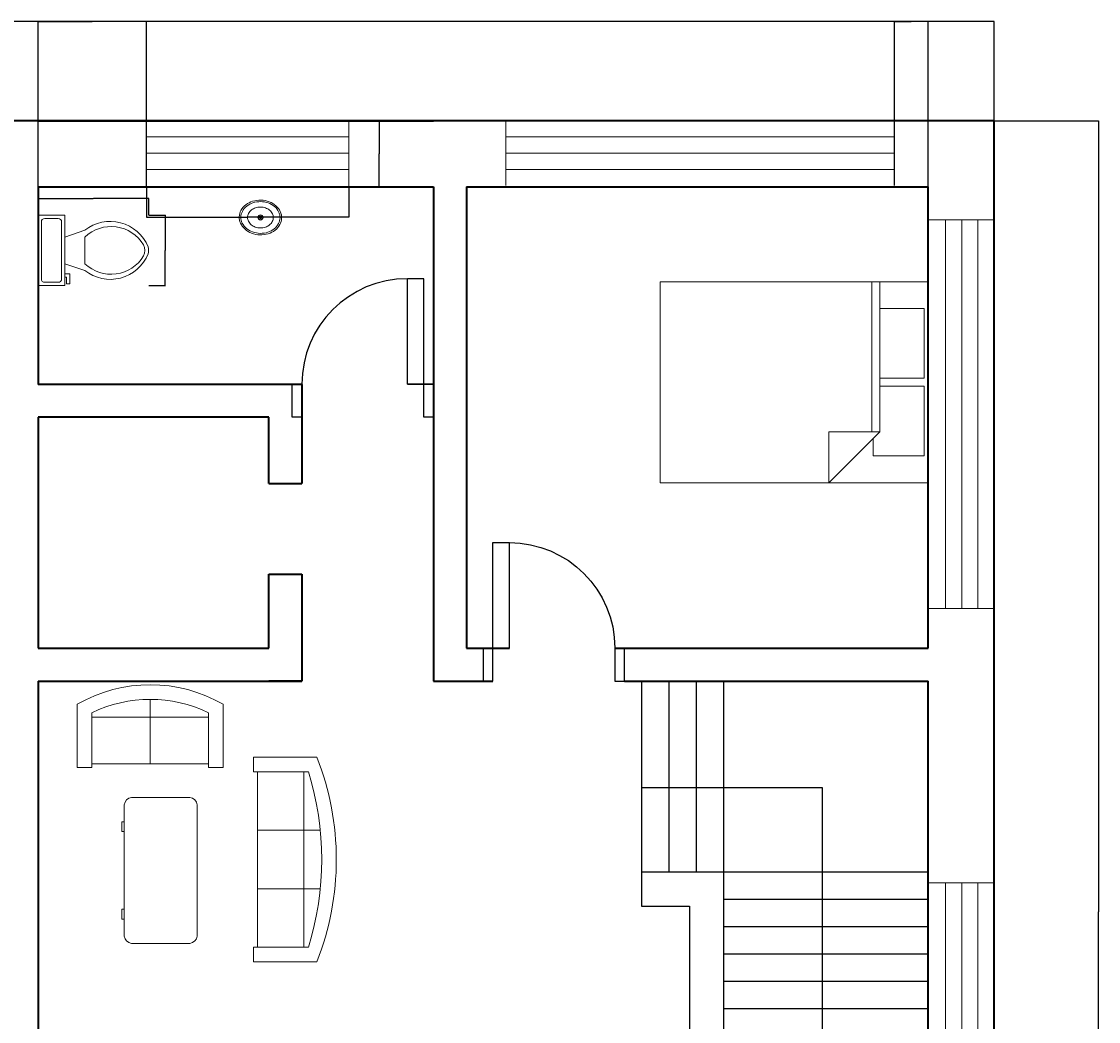
# Model space of a CAD drawing. Units: millimetres. Extents: x 726 to 37095, y -1634 to 13537.
# Tile 4 of 4: x 28928 to 37095, y 5952 to 13537. Entities that reach past the tile are written whole.
import ezdxf

# ---------------------------------------------------------------- set-up
doc = ezdxf.new("R2010")
doc.units = ezdxf.units.MM
for name, color, linetype, lineweight in [('A-ANNO-DIMS', 2, 'Continuous', 18), ('A-DOOR', 3, 'Continuous', 25), ('A-FLOR-FIXT', 9, 'Continuous', 18), ('A-FLOR-STRS', 5, 'Continuous', 25), ('A-FURN', 8, 'Continuous', 18), ('A-GLAZ', 4, 'Continuous', 18), ('A-WALL', 7, 'Continuous', 35)]:
    doc.layers.add(name, color=color, linetype=linetype, lineweight=lineweight)
doc.styles.get("Standard").update_dxf_attribs({"font": 'arial.ttf'})
doc.dimstyles.get("Standard").update_dxf_attribs({"dimtxt": 0.18, "dimasz": 0.18, "dimexe": 0.18, "dimexo": 0.0625, "dimgap": 0.09, "dimtad": 0, "dimtih": 1, "dimtoh": 1, "dimdec": 4, "dimzin": 0, "dimdsep": 46, "dimtxsty": 'Standard', "dimcen": 0.09, "dimadec": 0, "dimazin": 0, "dimtfac": 1, "dimtdec": 4, "dimtofl": 0, "dimtmove": 0, "dimatfit": 3, "dimfxl": 1, "dimtolj": 1, "dimtzin": 0, "dimarcsym": 0})

# ---------------------------------------------------------------- blocks, each defined once
blk = doc.blocks.new('Bed - Queen')
for p, q in [((0, -80.00003000000002), (0, 0)), ((0, 0), (59.99998999999999, 0)), ((59.99998999999999, 0), (59.99998999999999, -80.00003000000002)), ((7.99999, -1.200000000000017), (28.79998, -1.200000000000017)), ((7.99999, -14.4), (7.99999, -1.200000000000017)), ((28.79998, -1.200000000000017), (28.79998, -14.4)), ((31.19999, -1.200000000000017), (51.99999000000001, -1.200000000000017)), ((31.19999, -14.4), (31.19999, -1.200000000000017)), ((51.99999000000001, -1.200000000000017), (51.99999000000001, -16.4)), ((0, -14.4), (44.79999999999999, -14.4)), ((59.99998999999999, -29.60000000000001), (44.79999999999999, -14.4)), ((44.79999999999999, -14.4), (44.79999999999999, -29.60000000000001)), ((44.79999999999999, -16.80000000000001), (0, -16.80000000000001)), ((51.99999000000001, -16.4), (46.79936, -16.4)), ((44.79999999999999, -29.60000000000001), (59.99998999999999, -29.60000000000001)), ((59.99998999999999, -80.00003000000002), (0, -80.00003000000002))]:
    blk.add_line(p, q)
blk = doc.blocks.new('Window - Wood Frame 36 in. Wide plan')
for p, q in [((0, 6), (0, 0)), ((36, 6), (36, 0)), ((0, 4.5), (36, 4.5)), ((0, 3), (36, 3)), ((0, 1.5), (36, 1.5))]:
    blk.add_line(p, q)
blk = doc.blocks.new('Sofa - Roundback 7 ft.')
for p, q in [((-12.00002, -32.44210000000393), (-12.00003, -6.597100000003898)), ((11.99996999999999, -32.44210000000393), (11.99997999999999, -6.597100000003898)), ((-36.000027, -34.00000000000395), (-36.000027, -11.46960000000396)), ((35.99997999999999, -34.00000000000395), (35.99997999999999, -11.46960000000396)), ((-35.999844, -13.38190000000397), (35.99979999999999, -13.38190000000397)), ((-36.000027, -32.44210000000393), (35.99997999999999, -32.44210000000393))]:
    blk.add_line(p, q)
for points in [[(-36.000027, -34.00000000000395), (-42.000027, -34.00000000000395), (-42.000027, -8.000000000003944)], [(41.99997999999999, -8.000000000003944), (41.99997999999999, -34.00000000000395), (35.99997999999999, -34.00000000000395)]]:
    blk.add_lwpolyline(points)
for centre, radius, start, end in [((0, -114.2500000000039), 114.2500000000039, 68.43141000000072, 111.5686000000006), ((-1.00000000032e-05, -127.1968000000039), 121.1967999999973, 72.72032999999948, 107.2797000000005)]:
    blk.add_arc(centre, radius, start, end)
blk = doc.blocks.new('Desk - 30 x 60 in.')
for p, q in [((-26.999995, 0), (26.999995, 0)), ((-29.999995, -27), (-29.999995, -3)), ((29.999995, -3), (29.999995, -27)), ((26.999995, -30), (-26.999995, -30)), ((-20.000005, -30), (-20.000005, -31)), ((-16.000005, -31), (-16.000005, -30)), ((15.999995, -31), (15.999995, -30)), ((19.999995, -30), (19.999995, -31)), ((-20.000005, -31), (-16.000005, -31)), ((19.999995, -31), (15.999995, -31))]:
    blk.add_line(p, q)
for centre, radius, start, end in [((-26.499995, -3.5), 3.535534000004229, 98.1300999999916, 171.8698999999352), ((26.499995, -3.5), 3.535533999997753, 8.130102000022115, 81.8698999999439), ((-26.499995, -26.5), 3.535534000000845, 188.1301000000653, 261.8699000000085), ((26.499995, -26.5), 3.535534000004826, 278.1301000000561, 351.8698999999439)]:
    blk.add_arc(centre, radius, start, end)
blk = doc.blocks.new('Sofa - Roundback Loveseat 5 ft.')
for p, q in [((0, -32.44198000000246), (0, -5.999980000002448)), ((-23.99999999999999, -33.99998000000245), (-23.99999999999999, -11.46958000000243)), ((24.00004000000001, -33.99998000000245), (24.00004000000001, -11.46958000000243)), ((-23.99979999999998, -13.38178000000245), (23.99986, -13.38178000000245)), ((-23.99999999999999, -32.44198000000246), (24.00004000000001, -32.44198000000246))]:
    blk.add_line(p, q)
for points in [[(-23.99999999999999, -33.99998000000245), (-29.99999999999999, -33.99998000000245), (-29.99999999999999, -7.999980000002448)], [(30.00004000000001, -7.999980000002448), (30.00004000000001, -33.99998000000245), (24.00004000000001, -33.99998000000245)]]:
    blk.add_lwpolyline(points)
for centre, radius, start, end in [((0, -60.24998000000245), 60.24998000000245, 60.13715000000122, 119.862800000004), ((0, -61.38438000000245), 55.38444000000723, 64.32083000000306, 115.6791999999996)]:
    blk.add_arc(centre, radius, start, end)
blk = doc.blocks.new('Toilet - top')
for p, q in [((9.5, -6), (9.5, -2)), ((-10, -8.5), (-8, -8.5)), ((-10, -9.5), (-10, -8.5)), ((-7, -9.5), (-10, -9.5)), ((-8, -8.5), (-8, -8)), ((-7, -8), (-7, -9.5)), ((-4, -8), (-6, -14)), ((4, -8), (6, -14)), ((4, -14), (-4, -14))]:
    blk.add_line(p, q)
blk.add_lwpolyline([(10.5, -8), (10.5, 0), (-10.5, 0), (-10.5, -8)], close=True)
for points in [[(-9.5, -2), (-9.5, -6)], [(8.5, -1), (-8.5, -1)], [(-8.5, -7), (8.5, -7)]]:
    blk.add_lwpolyline(points)
for centre, radius, start, end in [((-8.625, -1.875), 0.8838834999999999, 81.86989999999999, 188.1301), ((8.625, -1.875), 0.8838834999999999, 351.8699, 98.13009999999998), ((-8.625, -6.125), 0.8838834999999999, 171.869898, 278.1301), ((8.625, -6.125), 0.8838834999999999, 261.8699, 8.130099999999993), ((3.519562435188956, -21.58049502388982), 12.16902005083646, 141.4691096810948, 247.9714346835576), ((4.199957580658807, -21.81740929088453), 11.3291791325804, 136.3677254423718, 238.946823937405), ((-3.519499936778316, -21.58047137067522), 12.16903423757823, 292.0284332733152, 38.53070636800453), ((-4.199890672038477, -21.81738596564128), 11.32918622148567, 301.0530065773863, 43.63209216694732), ((2.09660981727e-05, -27.87646475467881), 4, 245.7318247449371, 294.2681740488959), ((2.09415214183e-05, -28.99996806116075), 4, 254.8605283244437, 285.1394707718433)]:
    blk.add_arc(centre, radius, start, end)
blk = doc.blocks.new('Sink - Oval top')
for p, q in [((-1, 0), (1, 0)), ((0, 1), (0, -1))]:
    blk.add_line(p, q)
for points in [[(-12.23371880354079, 0.3941914712607968, 0.1176342565883263), (-11.46456229543957, -3.361933235489118, 0.104469279667093), (-8.878748691070427, -6.803541973650567, 0.0900157896014849), (-5.082757700676665, -9.072309807490512, 0.0819199491592185), (-0.3227280122732736, -10.01585280257211, 0.0819199491592091), (4.488169920880977, -9.380701564817912, 0.0900157896014801), (8.422342359155778, -7.36101289847943, 0.1044692796670922), (11.22435122606941, -4.093009071543406, 0.1176342565883338), (12.23371880354091, -0.3941914712607968, 0.1176342565883057), (11.46456229543992, 3.361933235488777, 0.1044692796670849), (8.878748691070427, 6.803541973650567, 0.0900157896014884), (5.082757700676324, 9.072309807490681, 0.0819199491592058), (0.3227280122732736, 10.01585280257211, 0.081919949159207), (-4.488169920880864, 9.380701564817969, 0.0900157896014802), (-8.422342359155778, 7.36101289847943, 0.1044692796670951), (-11.22435122606919, 4.093009071543633, 0.1176342565883402)], [(-11.28627986850119, 0.1590597164737346, 0.1186217001864142), (-10.51590095791209, -3.253161772358112, 0.1046781721811095), (-8.071803350560115, -6.358618019863342, 0.0895620664691738), (-4.537699193222351, -8.366971929609804, 0.0811846988912177), (-0.1289739026695997, -9.15150355811437, 0.0811846988912276), (4.300109150126218, -8.491524865184601, 0.0895620664691798), (7.889406708212618, -6.583562428127606, 0.1046781721811044), (10.42004782883111, -3.548216131892445, 0.1186217001864013), (11.28627986850119, -0.1590597164736209, 0.1186217001863945), (10.51590095791221, 3.253161772357998, 0.1046781721811069), (8.071803350560115, 6.358618019863342, 0.0895620664691756), (4.537699193222124, 8.366971929609917, 0.081184698891216), (0.1289739026695997, 9.151503558114428, 0.0811846988912142), (-4.300109150125877, 8.491524865184829, 0.0895620664691747), (-7.889406708212618, 6.583562428127606, 0.1046781721811045), (-10.42004782883111, 3.548216131892445, 0.1186217001863946)], [(-7.420452389032902, 0.0829876781601797, 0.1182825673856775), (-6.907065465214486, -2.1674649380775, 0.1046074595377274), (-5.294791470712084, -4.209988192029413, 0.0897179636260996), (-2.966599981142508, -5.528122152688069, 0.0814360825277113), (-0.0675135187855176, -6.036810076758797, 0.0814360825277218), (2.84222437824053, -5.593085960977873, 0.0897179636261315), (5.199312936802016, -4.327350491993342, 0.1046074595376878), (6.85686365682659, -2.321395784920355, 0.1182825673856714), (7.420452389033016, -0.0829876781601797, 0.1182825673856961), (6.907065465214486, 2.167464938077614, 0.1046074595377135), (5.294791470712084, 4.209988192029413, 0.0897179636261265), (2.966599981142621, 5.528122152687842, 0.0814360825277426), (0.0675135187855176, 6.036810076758797, 0.0814360825277225), (-2.842224378240644, 5.593085960977873, 0.0897179636261212), (-5.199312936802016, 4.327350491993342, 0.1046074595377049), (-6.856863656826476, 2.321395784920355, 0.1182825673856712)]]:
    blk.add_lwpolyline(points, format="xyb", close=True)
for radius in [1.5, 1]:
    blk.add_circle((0, 0), radius)
blk = doc.blocks.new('DOOR-SWING-800')
for p, q in [((999.1999999999979, 1050), (874.1999999999979, 1050)), ((874.1999999999979, 250), (874.1999999999979, 1050)), ((999.1999999999979, 250), (999.1999999999979, 1050)), ((9.095e-13, 250), (74.199999999998, 250)), ((9.095e-13, 0), (9.095e-13, 250)), ((74.199999999998, 250), (74.199999999998, 0)), ((874.1999999999979, 250), (999.1999999999979, 250)), ((999.1999999999979, 250), (1073.400000000002, 250)), ((999.1999999999979, 0), (999.1999999999979, 250)), ((1073.400000000002, 250), (1073.400000000002, 0)), ((74.199999999998, 0), (9.095e-13, 0)), ((1073.400000000002, 0), (999.1999999999979, 0))]:
    blk.add_line(p, q)
blk.add_arc((874.1999999999979, 250), 800, 90, 180)
blk = doc.blocks.new('STAIR-QUARTER-TURN')
for p, q in [((1551.94660387568, 5000.000000000002), (1551.94660387568, 3551.516503049365)), ((1758.872817725773, 5000.000000000002), (1758.872817725773, 3551.516503049365)), ((1965.799031575862, 5000.000000000002), (1965.799031575862, 3551.516503049365)), ((2172.725245425954, 5000.000000000002), (2172.725245425954, 3551.516503049365)), ((2172.725245425954, 4193.579423830473), (803.743340616409, 4193.579423830471)), ((803.743340616409, 4193.579423830471), (803.743340616409, 330.5564002077117)), ((2172.725245425954, 3551.516503049366), (0, 3551.516503049365)), ((1551.94660387568, 3551.516503049365), (1551.94660387568, 3344.590289199272)), ((2172.725245425954, 3551.516503049365), (2172.725245425954, 3292.858735736751)), ((1551.94660387568, 3344.590289199272), (0, 3344.590289199273)), ((1551.94660387568, 3344.590289199272), (1551.94660387568, 861.4757229981805)), ((2172.725245425954, 3292.858735736751), (1810.604371188295, 3292.858735736751)), ((1810.604371188295, 3292.85873573675), (1810.604371188295, 602.8179556856148)), ((1551.94660387568, 3137.664075349182), (0, 3137.664075349182)), ((1551.94660387568, 2930.73786149909), (0, 2930.737861499091)), ((1551.94660387568, 2723.811647649), (0, 2723.811647649001)), ((1551.94660387568, 2516.885433798908), (0, 2516.885433798909)), ((1551.94660387568, 2309.959219948817), (0, 2309.959219948818)), ((1551.94660387568, 2103.033006098726), (0, 2103.033006098727)), ((1551.94660387568, 1896.106792248635), (0, 1896.106792248635)), ((1551.94660387568, 1689.180578398543), (0, 1689.180578398544)), ((1551.94660387568, 1482.254364548453), (0, 1482.254364548454)), ((1551.94660387568, 1275.328150698362), (0, 1275.328150698363)), ((1551.94660387568, 1068.40193684827), (0, 1068.401936848271)), ((1551.94660387568, 861.4757229981795), (0, 861.4757229981805)), ((1551.94660387568, 861.4757229981805), (1551.946603875687, 602.8179556856074)), ((1810.604371188295, 602.8179556856148), (1551.946603875687, 602.8179556855675)), ((803.743340616409, 330.5564002077117), (545.0855733037969, 330.5564002077117)), ((545.0855733037969, 330.5564002077117), (803.743340616409, 4.547e-13)), ((803.743340616409, 330.5564002077117), (1062.401107929021, 330.5564002077108)), ((803.743340616409, 4.547e-13), (1062.401107929021, 330.5564002077117))]:
    blk.add_line(p, q)
blk = doc.blocks.new('WIN-1535')
for p, q in [((0, 1.819e-12), (0, 500.0000000000036)), ((1534.861597237876, 1.819e-12), (1534.861597237876, 500.0000000000036)), ((-9.095e-13, 377.1532172399693), (1534.861597237876, 377.1532172399693)), ((-9.095e-13, 254.306434479935), (1534.861597237876, 254.306434479935)), ((-9.095e-13, 131.459651719897), (1534.861597237876, 131.4596517198988))]:
    blk.add_line(p, q)
blk = doc.blocks.new('*D17')
at = {"layer": 'A-ANNO-DIMS', "color": 0, "lineweight": -2, "transparency": 16777216}
for p, q in [((29875.3043932246, 12283.82336812288), (29875.3043932246, 12053.4766285372)), ((31410.16599046248, 12283.82336812288), (31410.16599046248, 12053.4766285372)), ((29875.4843932246, 12053.6566285372), (30640.87736101134, 12053.6566285372)), ((31409.98599046248, 12053.6566285372), (30644.59302267573, 12053.6566285372))]:
    blk.add_line(p, q, dxfattribs=at)
at = {"layer": 'A-ANNO-DIMS', "color": 0, "transparency": 16777216}
for points in [[(29875.4843932246, 12053.6866285372), (29875.4843932246, 12053.6266285372), (29875.3043932246, 12053.6566285372)], [(31409.98599046248, 12053.6866285372), (31409.98599046248, 12053.6266285372), (31410.16599046248, 12053.6566285372)]]:
    blk.add_solid(points, dxfattribs=at)
at = {"layer": 'Defpoints', "color": 0, "transparency": 16777216}
for p in [(29875.3043932246, 12283.88586812288), (31410.16599046248, 12283.88586812288), (31410.16599046248, 12053.6566285372)]:
    blk.add_point(p, dxfattribs=at)
at = {"layer": 'A-ANNO-DIMS', "color": 0, "transparency": 16777216, "insert": (30642.73519184354, 12053.6566285372), "char_height": 0.18, "attachment_point": 5}
blk.add_mtext('\\A1;NARROW WINDOW 1535 TYP.', dxfattribs=at)
blk = doc.blocks.new('*D18')
at = {"layer": 'A-ANNO-DIMS', "color": 0, "lineweight": -2, "transparency": 16777216}
for p, q in [((31410.22849046249, 12783.88586812289), (31640.57523004819, 12783.88586812289)), ((31640.39523004819, 12783.70586812289), (31640.39523004819, 12534.06777126067)), ((31640.39523004819, 12284.06586812288), (31640.39523004819, 12533.7039649851)), ((31410.22849046249, 12283.88586812288), (31640.57523004819, 12283.88586812288))]:
    blk.add_line(p, q, dxfattribs=at)
at = {"layer": 'A-ANNO-DIMS', "color": 0, "transparency": 16777216}
for points in [[(31640.36523004819, 12783.70586812289), (31640.42523004819, 12783.70586812289), (31640.39523004819, 12783.88586812289)], [(31640.36523004819, 12284.06586812288), (31640.42523004819, 12284.06586812288), (31640.39523004819, 12283.88586812288)]]:
    blk.add_solid(points, dxfattribs=at)
at = {"layer": 'Defpoints', "color": 0, "transparency": 16777216}
for p in [(31410.16599046249, 12783.88586812289), (31640.39523004819, 12783.88586812289), (31410.16599046249, 12283.88586812288)]:
    blk.add_point(p, dxfattribs=at)
at = {"layer": 'A-ANNO-DIMS', "color": 0, "transparency": 16777216, "insert": (31640.39523004819, 12533.88586812287), "char_height": 0.18, "attachment_point": 5}
blk.add_mtext('\\A1;500 TYP.', dxfattribs=at)
blk = doc.blocks.new('*D31')
at = {"layer": 'A-ANNO-DIMS', "color": 0, "lineweight": -2, "transparency": 16777216}
for p, q in [((29053.40005351859, 12067.34836812288), (29053.40005351859, 12193.37205831405)), ((29053.58005351859, 12193.19205831405), (29472.24125592938, 12193.19205831405)), ((29892.59465479309, 12193.19205831405), (29473.93345238231, 12193.19205831405)), ((29892.77465479309, 12067.34836812288), (29892.77465479309, 12193.37205831405))]:
    blk.add_line(p, q, dxfattribs=at)
at = {"layer": 'A-ANNO-DIMS', "color": 0, "transparency": 16777216}
for points in [[(29053.58005351859, 12193.22205831405), (29053.58005351859, 12193.16205831405), (29053.40005351859, 12193.19205831405)], [(29892.59465479309, 12193.22205831405), (29892.59465479309, 12193.16205831405), (29892.77465479309, 12193.19205831405)]]:
    blk.add_solid(points, dxfattribs=at)
at = {"layer": 'Defpoints', "color": 0, "transparency": 16777216}
for p in [(29053.40005351859, 12193.19205831405), (29053.40005351859, 12067.28586812288), (29892.77465479309, 12067.28586812288)]:
    blk.add_point(p, dxfattribs=at)
at = {"layer": 'A-ANNO-DIMS', "color": 0, "transparency": 16777216, "insert": (29473.08735415584, 12193.19205831405), "char_height": 0.18, "attachment_point": 5}
blk.add_mtext('\\A1;WC 839 TYP.', dxfattribs=at)
blk = doc.blocks.new('*D32')
at = {"layer": 'A-ANNO-DIMS', "color": 0, "lineweight": -2, "transparency": 16777216}
for p, q in [((29892.8371547931, 12067.28586812288), (30018.86084498429, 12067.28586812288)), ((30018.68084498429, 12067.10586812288), (30018.68084498429, 11800.76783265221)), ((30018.68084498429, 11534.06586812288), (30018.68084498429, 11800.40390359355)), ((29892.8371547931, 11533.88586812288), (30018.86084498429, 11533.88586812288))]:
    blk.add_line(p, q, dxfattribs=at)
at = {"layer": 'A-ANNO-DIMS', "color": 0, "transparency": 16777216}
for points in [[(30018.65084498429, 12067.10586812288), (30018.71084498429, 12067.10586812288), (30018.68084498429, 12067.28586812288)], [(30018.65084498429, 11534.06586812288), (30018.71084498429, 11534.06586812288), (30018.68084498429, 11533.88586812288)]]:
    blk.add_solid(points, dxfattribs=at)
at = {"layer": 'Defpoints', "color": 0, "transparency": 16777216}
for p in [(29892.7746547931, 12067.28586812288), (30018.68084498429, 12067.28586812288), (29892.7746547931, 11533.88586812288)]:
    blk.add_point(p, dxfattribs=at)
at = {"layer": 'A-ANNO-DIMS', "color": 0, "transparency": 16777216, "insert": (30018.68084498429, 11800.58586812287), "char_height": 0.18, "attachment_point": 5}
blk.add_mtext('\\A1;533 TYP.', dxfattribs=at)
blk = doc.blocks.new('*D63')
at = {"layer": 'A-ANNO-DIMS', "color": 0, "lineweight": -2, "transparency": 16777216}
for p, q in [((21303.400054, 12783.948368), (21303.400054, 13536.815868)), ((21303.580054, 13536.635868), (28802.98013585539, 13536.635868)), ((36303.220054, 13536.635868), (28803.81997214461, 13536.635868)), ((36303.400054, 12783.948368), (36303.400054, 13536.815868))]:
    blk.add_line(p, q, dxfattribs=at)
at = {"layer": 'A-ANNO-DIMS', "color": 0, "transparency": 16777216}
for points in [[(21303.580054, 13536.665868), (21303.580054, 13536.605868), (21303.400054, 13536.635868)], [(36303.220054, 13536.665868), (36303.220054, 13536.605868), (36303.400054, 13536.635868)]]:
    blk.add_solid(points, dxfattribs=at)
at = {"layer": 'Defpoints', "color": 0, "transparency": 16777216}
for p in [(36303.400054, 13536.635868), (21303.400054, 12783.885868), (36303.400054, 12783.885868)]:
    blk.add_point(p, dxfattribs=at)
at = {"layer": 'A-ANNO-DIMS', "color": 0, "transparency": 16777216, "insert": (28803.400054, 13536.635868), "char_height": 0.18, "attachment_point": 5}
blk.add_mtext('\\A1;15000', dxfattribs=at)
blk = doc.blocks.new('*D64')
at = {"layer": 'A-ANNO-DIMS', "color": 0, "lineweight": -2, "transparency": 16777216}
for p, q in [((36303.46255400001, 12783.885868), (37094.80752400003, 12783.88586800001)), ((37094.62752400003, 12783.70586800001), (37094.62752400003, 6784.067771137793)), ((37094.62752400003, 784.065868000001), (37094.62752400003, 6783.703964862214)), ((32803.46255400001, 783.8858680000003), (37094.80752400003, 783.8858680000011))]:
    blk.add_line(p, q, dxfattribs=at)
at = {"layer": 'A-ANNO-DIMS', "color": 0, "transparency": 16777216}
for points in [[(37094.59752400003, 12783.70586800001), (37094.65752400003, 12783.70586800001), (37094.62752400003, 12783.88586800001)], [(37094.59752400003, 784.065868000001), (37094.65752400003, 784.065868000001), (37094.62752400003, 783.8858680000011)]]:
    blk.add_solid(points, dxfattribs=at)
at = {"layer": 'Defpoints', "color": 0, "transparency": 16777216}
for p in [(36303.40005400001, 12783.885868), (32803.40005400002, 783.8858680000003), (37094.62752400003, 783.8858680000011)]:
    blk.add_point(p, dxfattribs=at)
at = {"layer": 'A-ANNO-DIMS', "color": 0, "transparency": 16777216, "insert": (37094.62752400003, 6783.885867999991), "char_height": 0.18, "attachment_point": 5}
blk.add_mtext('\\A1;12000', dxfattribs=at)
blk = doc.blocks.new('*D75')
at = {"layer": 'A-ANNO-DIMS', "color": 0, "lineweight": -2, "transparency": 16777216}
for p, q in [((28553.400054, 12283.948368), (28553.400054, 13536.815868)), ((28553.580054, 13536.635868), (28803.11151375444, 13536.635868)), ((29053.220054, 13536.635868), (28803.68859424557, 13536.635868)), ((29053.400054, 12283.948368), (29053.400054, 13536.815868))]:
    blk.add_line(p, q, dxfattribs=at)
at = {"layer": 'A-ANNO-DIMS', "color": 0, "transparency": 16777216}
for points in [[(28553.580054, 13536.665868), (28553.580054, 13536.605868), (28553.400054, 13536.635868)], [(29053.220054, 13536.665868), (29053.220054, 13536.605868), (29053.400054, 13536.635868)]]:
    blk.add_solid(points, dxfattribs=at)
at = {"layer": 'Defpoints', "color": 0, "transparency": 16777216}
for p in [(29053.400054, 13536.635868), (28553.400054, 12283.885868), (29053.400054, 12283.885868)]:
    blk.add_point(p, dxfattribs=at)
at = {"layer": 'A-ANNO-DIMS', "color": 0, "transparency": 16777216, "insert": (28803.400054, 13536.635868), "char_height": 0.18, "attachment_point": 5}
blk.add_mtext('\\A1;500', dxfattribs=at)
blk = doc.blocks.new('*D77')
at = {"layer": 'A-ANNO-DIMS', "color": 0, "lineweight": -2, "transparency": 16777216}
for p, q in [((29053.400054, 12283.948368), (29053.400054, 13536.815868)), ((29053.580054, 13536.635868), (29463.95821258595, 13536.635868)), ((29875.124393, 13536.635868), (29464.74623441405, 13536.635868)), ((29875.304393, 12283.948368), (29875.304393, 13536.815868))]:
    blk.add_line(p, q, dxfattribs=at)
at = {"layer": 'A-ANNO-DIMS', "color": 0, "transparency": 16777216}
for points in [[(29053.580054, 13536.665868), (29053.580054, 13536.605868), (29053.400054, 13536.635868)], [(29875.124393, 13536.665868), (29875.124393, 13536.605868), (29875.304393, 13536.635868)]]:
    blk.add_solid(points, dxfattribs=at)
at = {"layer": 'Defpoints', "color": 0, "transparency": 16777216}
for p in [(29875.304393, 13536.635868), (29053.400054, 12283.885868), (29875.304393, 12283.885868)]:
    blk.add_point(p, dxfattribs=at)
at = {"layer": 'A-ANNO-DIMS', "color": 0, "transparency": 16777216, "insert": (29464.3522235, 13536.635868), "char_height": 0.18, "attachment_point": 5}
blk.add_mtext('\\A1;821.9', dxfattribs=at)
blk = doc.blocks.new('*D79')
at = {"layer": 'A-ANNO-DIMS', "color": 0, "lineweight": -2, "transparency": 16777216}
for p, q in [((35548.594604, 12292.561237), (35548.594604, 13536.815868)), ((35548.774604, 13536.635868), (35675.60190608049, 13536.635868)), ((35803.220054, 13536.635868), (35676.39275191951, 13536.635868)), ((35803.400054, 12283.948368), (35803.400054, 13536.815868))]:
    blk.add_line(p, q, dxfattribs=at)
at = {"layer": 'A-ANNO-DIMS', "color": 0, "transparency": 16777216}
for points in [[(35548.774604, 13536.665868), (35548.774604, 13536.605868), (35548.594604, 13536.635868)], [(35803.220054, 13536.665868), (35803.220054, 13536.605868), (35803.400054, 13536.635868)]]:
    blk.add_solid(points, dxfattribs=at)
at = {"layer": 'Defpoints', "color": 0, "transparency": 16777216}
for p in [(35803.400054, 13536.635868), (35548.594604, 12292.498737), (35803.400054, 12283.885868)]:
    blk.add_point(p, dxfattribs=at)
at = {"layer": 'A-ANNO-DIMS', "color": 0, "transparency": 16777216, "insert": (35675.997329, 13536.635868), "char_height": 0.18, "attachment_point": 5}
blk.add_mtext('\\A1;254.8', dxfattribs=at)

msp = doc.modelspace()

# ---------------------------------------------------------------- linework, layer by layer
at = {"layer": 'A-DOOR'}
for p, q in [((31979.20005351859, 11586.01711625042), (31854.20005351859, 11586.01711625042)), ((31854.20005351859, 10786.01711625042), (31854.20005351859, 11586.01711625042)), ((31979.20005351859, 10786.01711625042), (31979.20005351859, 11586.01711625042)), ((30980.00005351859, 10786.01711625042), (31054.20005351859, 10786.01711625042)), ((30980.00005351859, 10536.01711625042), (30980.00005351859, 10786.01711625042)), ((31054.20005351859, 10786.01711625042), (31054.20005351859, 10536.01711625042)), ((32053.40005351859, 10786.01711625042), (31854.20005351859, 10786.01711625042)), ((31854.20005351859, 10786.01711625042), (31979.20005351859, 10786.01711625042)), ((31979.20005351859, 10786.01711625042), (31854.20005351859, 10786.01711625042)), ((31979.20005351859, 10536.01711625042), (31979.20005351859, 10786.01711625042)), ((32053.40005351859, 10783.88586812288), (31979.20005351858, 10783.88586812288)), ((32053.40005351859, 10786.01711625042), (32053.40005351859, 10536.01711625042)), ((31054.20005351859, 10536.01711625042), (30980.00005351859, 10536.01711625042)), ((31054.20005351859, 10536.01711625042), (30980.00005351859, 10536.01711625042)), ((32053.40005351859, 10536.01711625042), (31979.20005351859, 10536.01711625042)), ((32428.40005351859, 8783.885868122885), (32428.40005351859, 8533.885868122885)), ((32502.6000535186, 8783.885868122885), (32627.6000535186, 8783.885868122885))]:
    msp.add_line(p, q, dxfattribs=at)
msp.add_arc((31854.20005351859, 10786.01711625042), 800, 90, 180, dxfattribs=at)
at = {"layer": 'A-FLOR-STRS'}
for p, q in [((33630.67480809263, 8533.885868122885), (33630.67480809263, 7085.402371172247)), ((33630.67480809263, 7085.402371172247), (33630.67480809263, 6826.744603859634))]:
    msp.add_line(p, q, dxfattribs=at)
at = {"layer": 'A-WALL'}
for p, q in [((36303.40005351859, 12783.88586812288), (21303.40005351859, 12783.88586812288)), ((29053.40005351859, 12783.88586812288), (32053.40005351859, 12783.88586812288)), ((36303.40005351859, 2283.885868122886), (36303.40005351859, 12783.88586812288)), ((29053.40005351859, 12283.88586812288), (29053.4000535186, 10783.88586812288)), ((29053.40005351859, 12283.88586812288), (32053.40005351859, 12283.88586812288)), ((32053.40005351859, 12283.88586812288), (32053.40005351859, 9283.885868122885)), ((32053.40005351859, 12283.88586812288), (32053.40005351859, 10783.88586812288)), ((32303.40005351859, 12283.88586812288), (32303.40005351859, 8783.885868122885)), ((32303.40005351859, 12283.88586812288), (35803.40005351859, 12283.88586812288)), ((35803.40005351859, 8783.885868122885), (35803.40005351859, 12283.88586812288)), ((31054.20005351859, 10783.88586812288), (29053.4000535186, 10783.88586812288)), ((31054.20005351859, 10783.88586812288), (31054.20005351859, 10032.95383072874)), ((29053.4000535186, 10536.01711625042), (29053.4000535186, 8783.885868122885)), ((30804.20005351859, 10536.01711625042), (29053.4000535186, 10536.01711625042)), ((30804.20005351859, 10032.95383072874), (30804.20005351859, 10536.01711625042)), ((30804.20005351858, 10032.95383072874), (31054.20005351859, 10032.95383072874)), ((30804.20005351859, 8783.885868122881), (30804.20005351859, 9345.861970410639)), ((30804.20005351858, 9345.861970410639), (31054.20005351859, 9345.861970410639)), ((31054.20005351859, 9345.861970410639), (31054.20005351859, 8533.885868122885)), ((32053.40005351859, 9283.885868122885), (32053.40005351859, 9033.885868122885)), ((32053.40005351859, 9033.885868122885), (32053.40005351859, 8783.885868122885)), ((29053.4000535186, 8783.885868122885), (30804.20005351858, 8783.885868122883)), ((32053.40005351859, 8783.885868122885), (32053.40005351859, 8533.885868122885)), ((32303.40005351859, 8783.885868122885), (32627.6000535186, 8783.885868122885)), ((33427.6000535186, 8783.885868122885), (35803.40005351859, 8783.885868122885)), ((29053.4000535186, 8533.885868122887), (31054.20005351859, 8533.885868122885)), ((29053.4000535186, 8533.885868122885), (29053.4000535186, 5033.885868122885)), ((31054.20005351859, 8533.885868122885), (30804.20005351859, 8533.885868122885)), ((32053.40005351859, 8533.885868122885), (32502.6000535186, 8533.885868122885)), ((33501.80005351859, 8533.885868122885), (33630.67480809263, 8533.885868122885)), ((33630.67480809263, 8533.885868122885), (35803.40005351859, 8533.885868122885)), ((35803.40005351859, 2783.885868122886), (35803.40005351859, 8533.885868122885))]:
    msp.add_line(p, q, dxfattribs=at)

# ---------------------------------------------------------------- block references
at = {"layer": 'A-DOOR', "extrusion": (0, 0, -1), "zscale": -1}
msp.add_blockref('DOOR-SWING-800', (-33501.80005351858, 8533.885868122878), dxfattribs=at)
at = {"layer": 'A-FLOR-FIXT', "xscale": 13.14744327818227, "yscale": 13.14744327818227, "zscale": 13.14744327818227}
msp.add_blockref('Sink - Oval top', (30740.00659218425, 12050.35577415071), dxfattribs=at)
at = {"layer": 'A-FLOR-FIXT', "xscale": 25.4, "yscale": 25.4, "zscale": 25.4, "rotation": 89.99999999999999}
msp.add_blockref('Toilet - top', (29053.40005351859, 11800.58586812288), dxfattribs=at)
at = {"layer": 'A-FLOR-STRS', "extrusion": (0, 0, -1), "zscale": -1}
msp.add_blockref('STAIR-QUARTER-TURN', (-35803.4000535186, 3533.885868122887), dxfattribs=at)
at = {"layer": 'A-FURN'}
for name, p, xscale, yscale, zscale, rotation in [('Bed - Queen', (35803.40005351859, 11562.56026255546), 25.4, 25.4, 25.4, 270), ('Sofa - Roundback 7 ft.', (31315.47765912056, 7180.161633685722), 18.46049527356076, 18.46049527356076, 18.46049527356076, 270.0000000000001), ('Desk - 30 x 60 in.', (30260.76707755922, 7097.540212527674), 18.46049527356076, 18.46049527356076, 18.46049527356076, 270.0000000000001)]:
    msp.add_blockref(name, p, dxfattribs=dict(at, xscale=xscale, yscale=yscale, zscale=zscale, rotation=rotation))
at = {"layer": 'A-FURN', "xscale": 18.46049527356076, "yscale": 18.46049527356076, "zscale": 18.46049527356076}
msp.add_blockref('Sofa - Roundback Loveseat 5 ft.', (29904.24581360826, 8505.704780616234), dxfattribs=at)
at = {"layer": 'A-GLAZ'}
msp.add_blockref('WIN-1535', (29875.3043932246, 12283.88586812288), dxfattribs=at)
at = {"layer": 'A-GLAZ', "xscale": 81.8978551733564, "yscale": 81.8978551733564, "zscale": 81.8978551733564}
msp.add_blockref('Window - Wood Frame 36 in. Wide plan', (32600.27181745432, 12292.49873708274), dxfattribs=at)
at = {"layer": 'A-GLAZ', "xscale": 81.8978551733564, "yscale": 81.8978551733564, "zscale": 81.8978551733564, "rotation": 270}
for p in [(35812.01292247846, 12031.35203741656), (35812.01292247845, 7003.139441062607)]:
    msp.add_blockref('Window - Wood Frame 36 in. Wide plan', p, dxfattribs=at)

# ---------------------------------------------------------------- dimensions: what is measured, and where the dimension line sits
at = {"layer": 'A-ANNO-DIMS'}
for base, p1, p2, override, picture, middle in [((36303.400054, 13536.635868), (21303.400054, 12783.885868), (36303.400054, 12783.885868), {"dimdec": 0, "dimlfac": 1, "dimrnd": 0, "dimzin": 0, "dimdsep": 46, "dimlunit": 2}, '*D63', (28803.400054, 13536.635868)), ((29053.400054, 13536.635868), (28553.400054, 12283.885868), (29053.400054, 12283.885868), {"dimdec": 0, "dimlfac": 1, "dimrnd": 0, "dimzin": 0, "dimdsep": 46, "dimlunit": 2}, '*D75', (28803.400054, 13536.635868)), ((29875.304393, 13536.635868), (29053.400054, 12283.885868), (29875.304393, 12283.885868), {"dimdec": 1, "dimlfac": 1, "dimrnd": 0, "dimzin": 0, "dimdsep": 46, "dimlunit": 2}, '*D77', (29464.3522235, 13536.635868)), ((35803.400054, 13536.635868), (35548.594604, 12292.498737), (35803.400054, 12283.885868), {"dimdec": 1, "dimlfac": 1, "dimrnd": 0, "dimzin": 0, "dimdsep": 46, "dimlunit": 2}, '*D79', (35675.997329, 13536.635868))]:
    dim = msp.add_linear_dim(base=base, p1=p1, p2=p2, dimstyle='Standard', override=override, dxfattribs=at)
    dim.commit()
    dim.dimension.update_dxf_attribs({"geometry": picture, "text_midpoint": middle})
for base, p1, p2, angle, text, picture, middle in [((31640.39523004819, 12783.88586812289), (31410.16599046248, 12283.88586812288), (31410.16599046248, 12783.88586812288), 90, '<> TYP.', '*D18', (31640.39523004819, 12533.88586812287)), ((29053.40005351859, 12193.19205831405), (29892.77465479309, 12067.28586812288), (29053.40005351859, 12067.28586812288), 179.9999999999998, 'WC <> TYP.', '*D31', (29473.08735415584, 12193.19205831405)), ((30018.68084498429, 12067.28586812288), (29892.77465479309, 11533.88586812288), (29892.77465479309, 12067.28586812288), 90, '<> TYP.', '*D32', (30018.68084498429, 11800.58586812287))]:
    dim = msp.add_linear_dim(base=base, p1=p1, p2=p2, angle=angle, text=text, dimstyle='Standard', override={"dimdec": 0, "dimlfac": 1, "dimrnd": 0, "dimzin": 0, "dimdsep": 46, "dimlunit": 2}, dxfattribs=at)
    dim.commit()
    dim.dimension.update_dxf_attribs({"geometry": picture, "text_midpoint": middle})
dim = msp.add_linear_dim(base=(37094.62752400003, 783.8858680000011), p1=(36303.400054, 12783.885868), p2=(32803.400054, 783.8858679999998), angle=90, dimstyle='Standard', override={"dimdec": 0, "dimlfac": 1, "dimrnd": 0, "dimzin": 0, "dimdsep": 46, "dimlunit": 2}, dxfattribs=at)
dim.commit()
dim.dimension.update_dxf_attribs({"geometry": '*D64', "text_midpoint": (37094.62752400003, 6783.885867999991)})
dim = msp.add_linear_dim(base=(31410.16599046248, 12053.6566285372), p1=(29875.3043932246, 12283.88586812288), p2=(31410.16599046248, 12283.88586812288), text='NARROW WINDOW <> TYP.', dimstyle='Standard', override={"dimdec": 0, "dimlfac": 1, "dimrnd": 0, "dimzin": 0, "dimdsep": 46, "dimlunit": 2}, dxfattribs=at)
dim.commit()
dim.dimension.update_dxf_attribs({"geometry": '*D17', "text_midpoint": (30642.73519184354, 12053.6566285372)})

doc.saveas('drawing.dxf')
